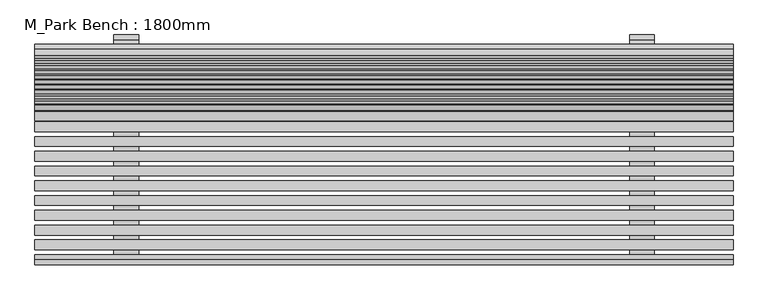
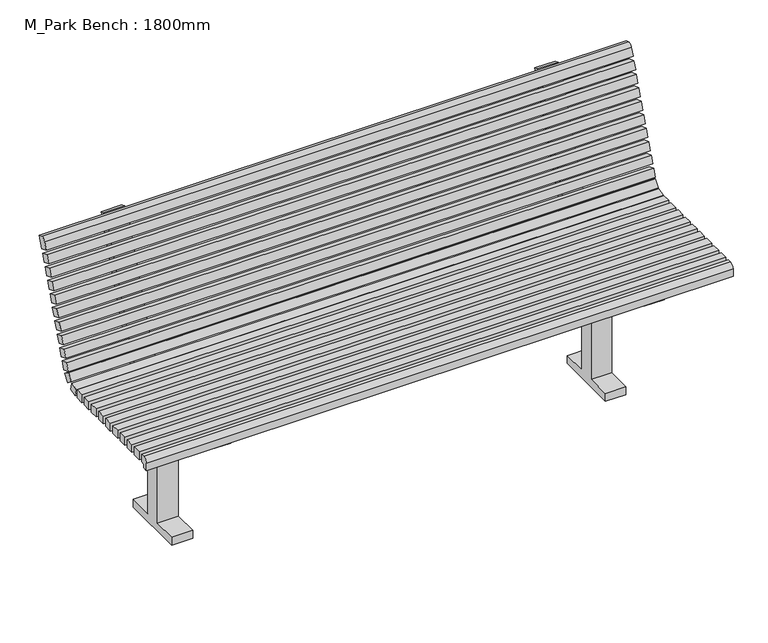
"""IFC4 building model written with IfcOpenShell, lengths in millimetres: geographic element geometry, M_Park Bench : 1800mm."""

from ifc_helpers import new_model, si_unit, point, frame, frame_2d, origin, place, context, project, spatial, polyline, circle_curve, trimmed, segment, composite_curve, outline, extrude, source, transform, mapped, element, save


def m_park_bench_1800mm_81f1f144(model_context):
    return source(origin(), model_context, "Body", "SweptSolid", [
        extrude(outline(composite_curve([segment(polyline([(-101.6, 25.4), (-25.4, 25.4), (-25.4, 431.8), (-304.8, 431.8), (-304.8, 457.2), (57.1368213, 457.2)]), True, "CONTINUOUS"), segment(trimmed(circle_curve(frame_2d((57.1368213, 520.7)), 63.5), [point((57.1368213, 457.2))], [point((116.8073027, 498.9817209))], True, "CARTESIAN"), True, "CONTINUOUS"), segment(polyline([(116.8073027, 498.9817209), (244.9406421, 851.0251774)]), True, "CONTINUOUS"), segment(trimmed(circle_curve(frame_2d((256.8747384, 846.6815216)), 12.7), [point((244.9406421, 851.0251774))], [point((261.2183942, 858.6156178))], False, "CARTESIAN"), True, "CONTINUOUS"), segment(polyline([(261.2183942, 858.6156178), (273.1524905, 854.271962), (140.6754953, 490.2944093)]), True, "CONTINUOUS"), segment(trimmed(circle_curve(frame_2d((57.1368213, 520.7)), 88.9), [point((140.6754953, 490.2944093))], [point((57.1368213, 431.8))], False, "CARTESIAN"), True, "CONTINUOUS"), segment(polyline([(57.1368213, 431.8), (25.4, 431.8), (25.4, 25.4), (101.6, 25.4), (101.6, 0.0), (-101.6, 0.0), (-101.6, 25.4)]), True, "CONTINUOUS")], self_intersect=False)), frame((-696.8, 0.0, 0.0), z_axis=(1.0, 0.0, 0.0), x_axis=(0.0, 1.0, 0.0)), (0.0, 0.0, 1.0), 63.8916859),
        extrude(outline(composite_curve([segment(polyline([(-101.6, 25.4), (-25.4, 25.4), (-25.4, 431.8), (-304.8, 431.8), (-304.8, 457.2), (57.1368213, 457.2)]), True, "CONTINUOUS"), segment(trimmed(circle_curve(frame_2d((57.1368213, 520.7)), 63.5), [point((57.1368213, 457.2))], [point((116.8073027, 498.9817209))], True, "CARTESIAN"), True, "CONTINUOUS"), segment(polyline([(116.8073027, 498.9817209), (244.9406421, 851.0251774)]), True, "CONTINUOUS"), segment(trimmed(circle_curve(frame_2d((256.8747384, 846.6815216)), 12.7), [point((244.9406421, 851.0251774))], [point((261.2183942, 858.6156178))], False, "CARTESIAN"), True, "CONTINUOUS"), segment(polyline([(261.2183942, 858.6156178), (273.1524905, 854.271962), (140.6754953, 490.2944093)]), True, "CONTINUOUS"), segment(trimmed(circle_curve(frame_2d((57.1368213, 520.7)), 88.9), [point((140.6754953, 490.2944093))], [point((57.1368213, 431.8))], False, "CARTESIAN"), True, "CONTINUOUS"), segment(polyline([(57.1368213, 431.8), (25.4, 431.8), (25.4, 25.4), (101.6, 25.4), (101.6, 0.0), (-101.6, 0.0), (-101.6, 25.4)]), True, "CONTINUOUS")], self_intersect=False)), frame((633.9736591, 0.0, 0.0), z_axis=(1.0, 0.0, 0.0), x_axis=(0.0, 1.0, 0.0)), (0.0, 0.0, 1.0), 62.8263409),
        extrude(outline(polyline([(900.0, -255.4337104), (900.0, -280.8337104), (-900.0, -280.8337104), (-900.0, -255.4337104), (900.0, -255.4337104)])), frame((0.0, 0.0, 457.2), z_axis=(0.0, 0.0, 1.0), x_axis=(1.0, 0.0, 0.0)), (0.0, 0.0, 1.0), 25.4),
        extrude(outline(polyline([(900.0, -217.3337104), (900.0, -242.7337104), (-900.0, -242.7337104), (-900.0, -217.3337104), (900.0, -217.3337104)])), frame((0.0, 0.0, 457.2), z_axis=(0.0, 0.0, 1.0), x_axis=(1.0, 0.0, 0.0)), (0.0, 0.0, 1.0), 25.4),
        extrude(outline(polyline([(900.0, -179.2337104), (900.0, -204.6337104), (-900.0, -204.6337104), (-900.0, -179.2337104), (900.0, -179.2337104)])), frame((0.0, 0.0, 457.2), z_axis=(0.0, 0.0, 1.0), x_axis=(1.0, 0.0, 0.0)), (0.0, 0.0, 1.0), 25.4),
        extrude(outline(polyline([(900.0, -141.1337104), (900.0, -166.5337104), (-900.0, -166.5337104), (-900.0, -141.1337104), (900.0, -141.1337104)])), frame((0.0, 0.0, 457.2), z_axis=(0.0, 0.0, 1.0), x_axis=(1.0, 0.0, 0.0)), (0.0, 0.0, 1.0), 25.4),
        extrude(outline(polyline([(900.0, -103.0337104), (900.0, -128.4337104), (-900.0, -128.4337104), (-900.0, -103.0337104), (900.0, -103.0337104)])), frame((0.0, 0.0, 457.2), z_axis=(0.0, 0.0, 1.0), x_axis=(1.0, 0.0, 0.0)), (0.0, 0.0, 1.0), 25.4),
        extrude(outline(polyline([(900.0, -64.9337104), (900.0, -90.3337104), (-900.0, -90.3337104), (-900.0, -64.9337104), (900.0, -64.9337104)])), frame((0.0, 0.0, 457.2), z_axis=(0.0, 0.0, 1.0), x_axis=(1.0, 0.0, 0.0)), (0.0, 0.0, 1.0), 25.4),
        extrude(outline(polyline([(900.0, -26.8337104), (900.0, -52.2337104), (-900.0, -52.2337104), (-900.0, -26.8337104), (900.0, -26.8337104)])), frame((0.0, 0.0, 457.2), z_axis=(0.0, 0.0, 1.0), x_axis=(1.0, 0.0, 0.0)), (0.0, 0.0, 1.0), 25.4),
        extrude(outline(polyline([(900.0, 11.2662896), (900.0, -14.1337104), (-900.0, -14.1337104), (-900.0, 11.2662896), (900.0, 11.2662896)])), frame((0.0, 0.0, 457.2), z_axis=(0.0, 0.0, 1.0), x_axis=(1.0, 0.0, 0.0)), (0.0, 0.0, 1.0), 25.4),
        extrude(outline(polyline([(900.0, 49.3662896), (900.0, 23.9662896), (-900.0, 23.9662896), (-900.0, 49.3662896), (900.0, 49.3662896)])), frame((0.0, 0.0, 457.2), z_axis=(0.0, 0.0, 1.0), x_axis=(1.0, 0.0, 0.0)), (0.0, 0.0, 1.0), 25.4),
        extrude(outline(composite_curve([segment(polyline([(-304.8, 457.2), (-304.8, 444.5), (-318.9337104, 444.5), (-318.9337104, 468.3125)]), True, "CONTINUOUS"), segment(trimmed(circle_curve(frame_2d((-304.6462104, 468.3125)), 14.2875), [point((-318.9337104, 468.3125))], [point((-304.6462104, 482.6))], False, "CARTESIAN"), True, "CONTINUOUS"), segment(polyline([(-304.6462104, 482.6), (-293.5337104, 482.6), (-293.5337104, 457.2), (-304.8, 457.2)]), True, "CONTINUOUS")], self_intersect=False)), frame((-900.0, 0.0, 0.0), z_axis=(1.0, 0.0, 0.0), x_axis=(0.0, 1.0, 0.0)), (0.0, 0.0, 1.0), 1800.0),
        extrude(outline(polyline([(0.0, -25.4), (0.0, 0.0), (1800.0, 0.0), (1800.0, -25.4), (0.0, -25.4)])), frame((900.0, 121.2738625, 585.5181247), z_axis=(0.0, 0.342020143325687, 0.9396926207859018), x_axis=(-1.0, 0.0, 0.0)), (0.0, 0.0, 1.0), 25.4),
        extrude(outline(polyline([(0.0, -25.4), (0.0, 0.0), (1800.0, 0.0), (1800.0, -25.4), (0.0, -25.4)])), frame((900.0, 134.30483, 621.3204136), z_axis=(0.0, 0.34202014332568254, 0.9396926207859034), x_axis=(-1.0, 0.0, 0.0)), (0.0, 0.0, 1.0), 25.4),
        extrude(outline(polyline([(0.0, -25.3999999), (0.0, 0.0), (1800.0, 0.0), (1800.0, -25.3999999), (0.0, -25.3999999)])), frame((900.0, 95.2119276, 513.913547), z_axis=(0.0, 0.34202014332568254, 0.9396926207859034), x_axis=(-1.0, 0.0, 0.0)), (0.0, 0.0, 1.0), 25.4),
        extrude(outline(polyline([(0.0, -25.4000001), (0.0, 0.0), (1800.0, 0.0), (1800.0, -25.4000001), (0.0, -25.4000001)])), frame((900.0, 108.242895, 549.7158359), z_axis=(0.0, 0.34202014332567804, 0.9396926207859051), x_axis=(-1.0, 0.0, 0.0)), (0.0, 0.0, 1.0), 25.4),
        extrude(outline(polyline([(0.0, -25.4), (0.0, 0.0), (1800.0, 0.0), (1800.0, -25.4), (0.0, -25.4)])), frame((900.0, 173.3977323, 728.7272801), z_axis=(0.0, 0.34202014332568337, 0.9396926207859031), x_axis=(-1.0, 0.0, 0.0)), (0.0, 0.0, 1.0), 25.4),
        extrude(outline(polyline([(0.0, -25.4000001), (0.0, 0.0), (1800.0, 0.0), (1800.0, -25.4000001), (0.0, -25.4000001)])), frame((900.0, 186.4286998, 764.529569), z_axis=(0.0, 0.3420201433256829, 0.9396926207859032), x_axis=(-1.0, 0.0, 0.0)), (0.0, 0.0, 1.0), 25.4),
        extrude(outline(polyline([(0.0, -25.4), (0.0, 0.0), (1800.0, 0.0), (1800.0, -25.4), (0.0, -25.4)])), frame((900.0, 147.3357974, 657.1227024), z_axis=(0.0, 0.3420201433256776, 0.9396926207859052), x_axis=(-1.0, 0.0, 0.0)), (0.0, 0.0, 1.0), 25.4),
        extrude(outline(polyline([(0.0, -25.4), (0.0, 0.0), (1800.0, 0.0), (1800.0, -25.4), (0.0, -25.4)])), frame((900.0, 160.3667649, 692.9249913), z_axis=(0.0, 0.34202014332568254, 0.9396926207859034), x_axis=(-1.0, 0.0, 0.0)), (0.0, 0.0, 1.0), 25.4),
        extrude(outline(polyline([(0.0, -25.3999999), (0.0, 0.0), (1800.0, 0.0), (1800.0, -25.3999999), (0.0, -25.3999999)])), frame((900.0, 199.4596673, 800.3318578), z_axis=(0.0, 0.3420201433256774, 0.9396926207859052), x_axis=(-1.0, 0.0, 0.0)), (0.0, 0.0, 1.0), 25.4),
        extrude(outline(composite_curve([segment(polyline([(249.3897948, 863.2491239), (236.3588273, 827.4468351), (212.4906347, 836.1341467), (221.1779464, 860.0023393)]), True, "CONTINUOUS"), segment(trimmed(circle_curve(frame_2d((233.1120426, 855.6586834)), 12.7), [point((221.1779464, 860.0023393))], [point((237.4556985, 867.5927797))], False, "CARTESIAN"), True, "CONTINUOUS"), segment(polyline([(237.4556985, 867.5927797), (249.3897948, 863.2491239)]), True, "CONTINUOUS")], self_intersect=False)), frame((-900.0, 0.0, 0.0), z_axis=(1.0, 0.0, 0.0), x_axis=(0.0, 1.0, 0.0)), (0.0, 0.0, 1.0), 1800.0),
        extrude(outline(polyline([(0.0, -25.4), (0.0, 0.0), (1800.0, 0.0), (1800.0, -25.4), (0.0, -25.4)])), frame((900.0, 78.7855779, 490.7267336), z_axis=(0.0, 0.5735764363510742, 0.8191520442889721), x_axis=(-1.0, 0.0, 0.0)), (0.0, 0.0, 1.0), 25.4),
        extrude(outline(polyline([(0.0, -25.4), (0.0, 0.0), (1800.0, 0.0), (1800.0, -25.4), (0.0, -25.4)])), frame((900.0, 59.0817015, 457.2297909), z_axis=(0.0, -0.2588190451024684, 0.9659258262890824), x_axis=(-1.0, 0.0, 0.0)), (0.0, 0.0, 1.0), 25.4),
    ])


if __name__ == "__main__":
    model = new_model("IFC4")
    model_context = context("Model", 3, world=origin())
    ifc_project = project(units=[si_unit("LENGTHUNIT", "METRE", prefix="MILLI")], contexts=[model_context])
    site = spatial("IfcSite", under=ifc_project)
    building = spatial("IfcBuilding", under=site)
    placement = place(None, origin())
    m_park_bench_1800mm_shape = m_park_bench_1800mm_81f1f144(model_context)
    element("IfcGeographicElement", 1, ObjectType="M_Park Bench : 1800mm", at=placement, inside=building, context=model_context, shape_type="MappedRepresentation", body=[
        mapped(m_park_bench_1800mm_shape, transform((0.0, 0.0, 0.0), x_axis=(1.0, 0.0, 0.0), y_axis=(0.0, 1.0, 0.0), z_axis=(0.0, 0.0, 1.0))),
    ])
    save(model, "model.ifc")

# Revit data of these elements
# Type "M_Park Bench : 1800mm"
#   Length = 5' - 10.86614"
#   Seat Material = Wood - Teak
#   Frame Material = Steel, Paint Finish, Dark Gray, Matte
# Element 1 (IfcGeographicElement, "M_Park Bench : 1800mm")
#   Materials on its faces: "Wood - Teak", "Steel, Paint Finish, Dark Gray, Matte"
# Materials
#   "Wood - Teak": class "Wood", colour RGB 120 73 19, transparency 0
#   "Steel, Paint Finish, Dark Gray, Matte": class "Metal", colour RGB 98 98 98, transparency 0, Description = "Steel, paint finish, dark gray, matte", Cost = 0
